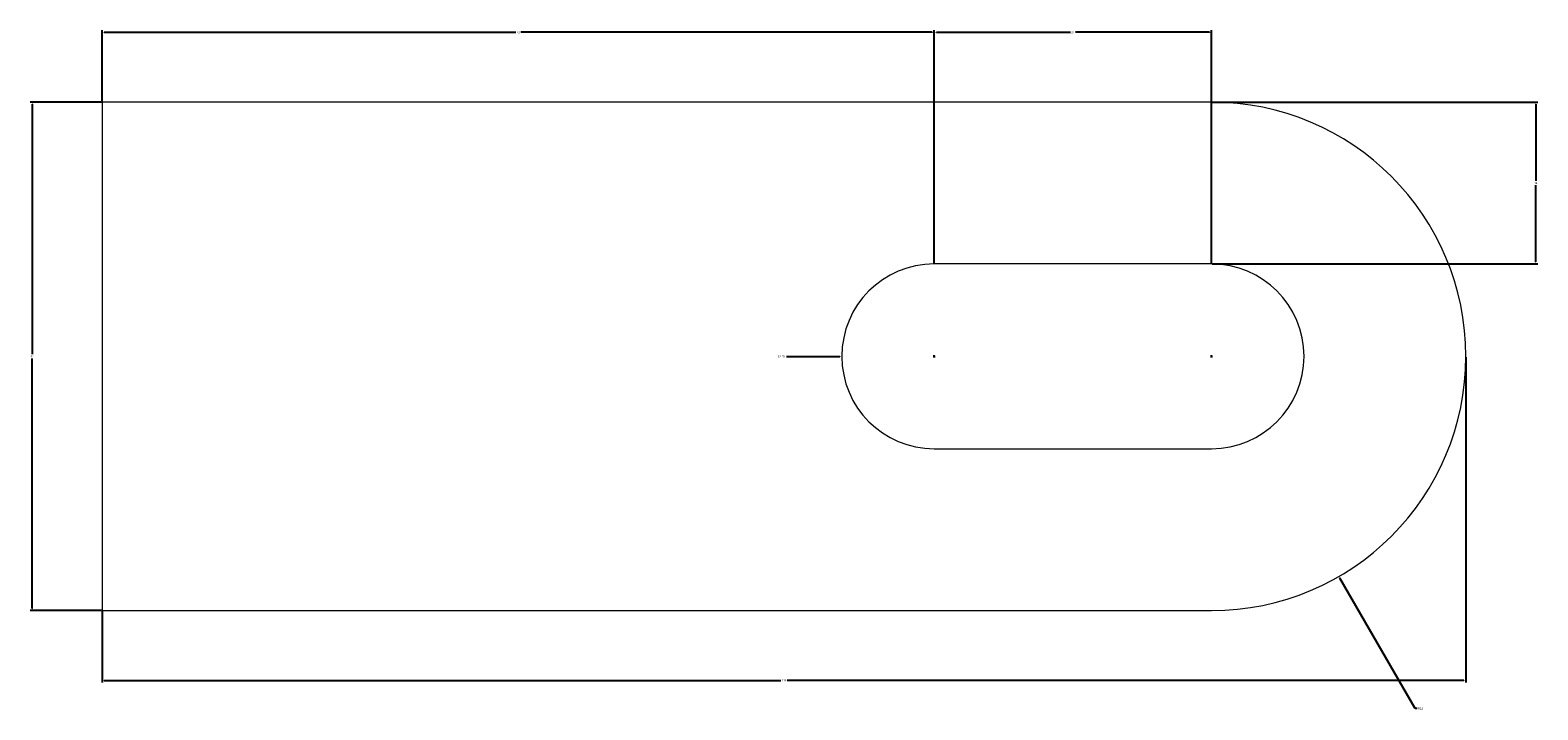
# Model space of a CAD drawing. Units: millimetres. Extents: x 3613 to 3838, y -3 to 1390.
# Tile 2 of 2: x 3613 to 3744, y 1331 to 1390. Entities that reach past the tile are written whole.
import ezdxf

# ---------------------------------------------------------------- set-up
doc = ezdxf.new("R2010")
doc.units = ezdxf.units.MM
doc.layers.add('M-CONS', color=7, linetype='Continuous', lineweight=18)
doc.layers.add('M-DIMS', color=2, linetype='Continuous', lineweight=18)
doc.styles.get("Standard").update_dxf_attribs({"font": 'arial.ttf'})
doc.dimstyles.get("Standard").update_dxf_attribs({"dimtxt": 0.18, "dimasz": 0.18, "dimexe": 0.18, "dimexo": 0.0625, "dimgap": 0.09, "dimtad": 0, "dimtih": 1, "dimtoh": 1, "dimdec": 4, "dimzin": 0, "dimdsep": 46, "dimtxsty": 'Standard', "dimcen": 0.09, "dimadec": 0, "dimazin": 0, "dimtfac": 1, "dimtdec": 4, "dimtofl": 0, "dimtmove": 0, "dimatfit": 3, "dimfxl": 1, "dimtolj": 1, "dimtzin": 0, "dimarcsym": 0})

# ---------------------------------------------------------------- blocks, each defined once
blk = doc.blocks.new('*D1')
at = {"layer": 'Defpoints', "color": 0, "transparency": 16777216}
for p in [(3737.71, 1361.28), (3619.71, 1339.28), (3737.71, 1333.23)]:
    blk.add_point(p, dxfattribs=at)
at = {"layer": 'M-DIMS', "color": 0, "lineweight": -2, "transparency": 16777216}
for p, q in [((3737.71, 1361.22), (3737.71, 1333.05)), ((3619.71, 1339.22), (3619.71, 1333.05)), ((3619.89, 1333.23), (3678.43, 1333.23)), ((3737.53, 1333.23), (3678.99, 1333.23))]:
    blk.add_line(p, q, dxfattribs=at)
at = {"layer": 'M-DIMS', "color": 0, "transparency": 16777216}
for points in [[(3619.89, 1333.26), (3619.89, 1333.2), (3619.71, 1333.23)], [(3737.53, 1333.26), (3737.53, 1333.2), (3737.71, 1333.23)]]:
    blk.add_solid(points, dxfattribs=at)
at = {"layer": 'M-DIMS', "color": 0, "transparency": 16777216, "insert": (3678.71, 1333.23), "char_height": 0.18, "attachment_point": 5}
blk.add_mtext('\\A1;118', dxfattribs=at)
blk = doc.blocks.new('*D2')
at = {"layer": 'Defpoints', "color": 0, "transparency": 16777216}
for p in [(3613.65792, 1383.283895), (3619.70792, 1383.283895), (3619.70792, 1339.283895)]:
    blk.add_point(p, dxfattribs=at)
at = {"layer": 'M-DIMS', "color": 0, "lineweight": -2, "transparency": 16777216}
for p, q in [((3619.64542, 1383.283895), (3613.47792, 1383.283895)), ((3613.65792, 1383.103895), (3613.65792, 1361.463895)), ((3613.65792, 1339.463895), (3613.65792, 1361.103895)), ((3619.64542, 1339.283895), (3613.47792, 1339.283895))]:
    blk.add_line(p, q, dxfattribs=at)
at = {"layer": 'M-DIMS', "color": 0, "transparency": 16777216}
for points in [[(3613.62792, 1383.103895), (3613.68792, 1383.103895), (3613.65792, 1383.283895)], [(3613.62792, 1339.463895), (3613.68792, 1339.463895), (3613.65792, 1339.283895)]]:
    blk.add_solid(points, dxfattribs=at)
at = {"layer": 'M-DIMS', "color": 0, "transparency": 16777216, "insert": (3613.65792, 1361.283895), "char_height": 0.18, "attachment_point": 5}
blk.add_mtext('\\A1;44', dxfattribs=at)
blk = doc.blocks.new('*D3')
at = {"layer": 'Defpoints', "color": 0, "transparency": 16777216}
for p in [(3715.71, 1389.33), (3691.71, 1369.28), (3715.71, 1369.28)]:
    blk.add_point(p, dxfattribs=at)
at = {"layer": 'M-DIMS', "color": 0, "lineweight": -2, "transparency": 16777216}
for p, q in [((3691.71, 1369.35), (3691.71, 1389.51)), ((3715.71, 1369.35), (3715.71, 1389.51)), ((3691.89, 1389.33), (3703.49, 1389.33)), ((3715.53, 1389.33), (3703.93, 1389.33))]:
    blk.add_line(p, q, dxfattribs=at)
at = {"layer": 'M-DIMS', "color": 0, "transparency": 16777216}
for points in [[(3691.89, 1389.36), (3691.89, 1389.3), (3691.71, 1389.33)], [(3715.53, 1389.36), (3715.53, 1389.3), (3715.71, 1389.33)]]:
    blk.add_solid(points, dxfattribs=at)
at = {"layer": 'M-DIMS', "color": 0, "transparency": 16777216, "insert": (3703.71, 1389.33), "char_height": 0.18, "attachment_point": 5}
blk.add_mtext('\\A1;24', dxfattribs=at)
blk = doc.blocks.new('*D4')
at = {"layer": 'Defpoints', "color": 0, "transparency": 16777216}
for p in [(3715.71, 1383.28), (3743.76, 1383.28), (3715.71, 1369.28)]:
    blk.add_point(p, dxfattribs=at)
at = {"layer": 'M-DIMS', "color": 0, "lineweight": -2, "transparency": 16777216}
for p, q in [((3715.77, 1383.28), (3743.94, 1383.28)), ((3743.76, 1383.1), (3743.76, 1376.46)), ((3743.76, 1369.46), (3743.76, 1376.1)), ((3715.77, 1369.28), (3743.94, 1369.28))]:
    blk.add_line(p, q, dxfattribs=at)
at = {"layer": 'M-DIMS', "color": 0, "transparency": 16777216}
for points in [[(3743.73, 1383.1), (3743.79, 1383.1), (3743.76, 1383.28)], [(3743.73, 1369.46), (3743.79, 1369.46), (3743.76, 1369.28)]]:
    blk.add_solid(points, dxfattribs=at)
at = {"layer": 'M-DIMS', "color": 0, "transparency": 16777216, "insert": (3743.76, 1376.28), "char_height": 0.18, "attachment_point": 5}
blk.add_mtext('\\A1;14', dxfattribs=at)
blk = doc.blocks.new('*D5')
at = {"layer": 'Defpoints', "color": 0, "transparency": 16777216}
for p in [(3691.71, 1389.33), (3619.71, 1383.28), (3691.71, 1369.28)]:
    blk.add_point(p, dxfattribs=at)
at = {"layer": 'M-DIMS', "color": 0, "lineweight": -2, "transparency": 16777216}
for p, q in [((3619.71, 1383.35), (3619.71, 1389.51)), ((3691.71, 1369.35), (3691.71, 1389.51)), ((3619.89, 1389.33), (3655.49, 1389.33)), ((3691.53, 1389.33), (3655.93, 1389.33))]:
    blk.add_line(p, q, dxfattribs=at)
at = {"layer": 'M-DIMS', "color": 0, "transparency": 16777216}
for points in [[(3619.89, 1389.36), (3619.89, 1389.3), (3619.71, 1389.33)], [(3691.53, 1389.36), (3691.53, 1389.3), (3691.71, 1389.33)]]:
    blk.add_solid(points, dxfattribs=at)
at = {"layer": 'M-DIMS', "color": 0, "transparency": 16777216, "insert": (3655.71, 1389.33), "char_height": 0.18, "attachment_point": 5}
blk.add_mtext('\\A1;72', dxfattribs=at)
blk = doc.blocks.new('*D7')
at = {"layer": 'Defpoints', "color": 0, "transparency": 16777216}
for p in [(3715.71, 1361.28), (3726.71, 1342.23)]:
    blk.add_point(p, dxfattribs=at)
at = {"layer": 'M-DIMS', "color": 0, "lineweight": -2, "transparency": 16777216}
for p, q in [((3715.62, 1361.28), (3715.8, 1361.28)), ((3715.71, 1361.19), (3715.71, 1361.37)), ((3733.31, 1330.8), (3726.8, 1342.08)), ((3733.49, 1330.8), (3733.31, 1330.8))]:
    blk.add_line(p, q, dxfattribs=at)
at = {"layer": 'M-DIMS', "color": 0, "transparency": 16777216}
blk.add_solid([(3726.82, 1342.09), (3726.77, 1342.06), (3726.71, 1342.23)], dxfattribs=at)
at = {"layer": 'M-DIMS', "color": 0, "transparency": 16777216, "insert": (3733.79, 1330.8), "char_height": 0.18, "attachment_point": 5}
blk.add_mtext('\\A1;R22', dxfattribs=at)
blk = doc.blocks.new('*D8')
at = {"layer": 'Defpoints', "color": 0, "transparency": 16777216}
for p in [(3683.71, 1361.28), (3691.71, 1361.28)]:
    blk.add_point(p, dxfattribs=at)
at = {"layer": 'M-DIMS', "color": 0, "lineweight": -2, "transparency": 16777216}
for p, q in [((3678.91, 1361.28), (3683.53, 1361.28)), ((3691.62, 1361.28), (3691.8, 1361.28)), ((3691.71, 1361.19), (3691.71, 1361.37))]:
    blk.add_line(p, q, dxfattribs=at)
at = {"layer": 'M-DIMS', "color": 0, "transparency": 16777216}
blk.add_solid([(3683.53, 1361.31), (3683.53, 1361.25), (3683.71, 1361.28)], dxfattribs=at)
at = {"layer": 'M-DIMS', "color": 0, "transparency": 16777216, "insert": (3678.48, 1361.28), "char_height": 0.18, "attachment_point": 5}
blk.add_mtext('\\A1;2X R8', dxfattribs=at)

msp = doc.modelspace()

# ---------------------------------------------------------------- linework, layer by layer
at = {"layer": 'M-CONS'}
for points in [[(3715.71, 1383.28), (3619.71, 1383.28), (3619.71, 1339.28), (3715.71, 1339.28, 1)], [(3715.71, 1369.28), (3691.71, 1369.28, 1), (3691.71, 1353.28), (3715.71, 1353.28, 1)]]:
    msp.add_lwpolyline(points, format="xyb", close=True, dxfattribs=at)

# ---------------------------------------------------------------- dimensions: what is measured, and where the dimension line sits
at = {"layer": 'M-DIMS'}
for base, p1, p2, picture, middle in [((3691.71, 1389.33), (3619.71, 1383.28), (3691.71, 1369.28), '*D5', (3655.71, 1389.33)), ((3715.71, 1389.33), (3691.71, 1369.28), (3715.71, 1369.28), '*D3', (3703.71, 1389.33)), ((3737.71, 1333.23), (3619.71, 1339.28), (3737.71, 1361.28), '*D1', (3678.71, 1333.23))]:
    dim = msp.add_linear_dim(base=base, p1=p1, p2=p2, dimstyle='Standard', override={"dimdec": 0, "dimlfac": 1, "dimrnd": 0, "dimzin": 0, "dimdsep": 46, "dimlunit": 2}, dxfattribs=at)
    dim.commit()
    dim.dimension.update_dxf_attribs({"geometry": picture, "text_midpoint": middle})
for base, p1, p2, picture, middle in [((3613.66, 1383.28), (3619.71, 1339.28), (3619.71, 1383.28), '*D2', (3613.66, 1361.28)), ((3743.76, 1383.28), (3715.71, 1369.28), (3715.71, 1383.28), '*D4', (3743.76, 1376.28))]:
    dim = msp.add_linear_dim(base=base, p1=p1, p2=p2, angle=90, dimstyle='Standard', override={"dimdec": 0, "dimlfac": 1, "dimrnd": 0, "dimzin": 0, "dimdsep": 46, "dimlunit": 2}, dxfattribs=at)
    dim.commit()
    dim.dimension.update_dxf_attribs({"geometry": picture, "text_midpoint": middle})
dim = msp.add_radius_dim(center=(3691.71, 1361.28), mpoint=(3683.71, 1361.28), text='2X <>', dimstyle='Standard', override={"dimdec": 0, "dimlfac": 1, "dimrnd": 0, "dimzin": 0, "dimdsep": 46, "dimlunit": 2}, dxfattribs=at)
dim.commit()
dim.dimension.update_dxf_attribs({"geometry": '*D8', "text_midpoint": (3678.91, 1361.28), "dimtype": 164})
dim = msp.add_radius_dim(center=(3715.71, 1361.28), mpoint=(3726.71, 1342.23), dimstyle='Standard', override={"dimdec": 0, "dimlfac": 1, "dimrnd": 0, "dimzin": 0, "dimdsep": 46, "dimlunit": 2}, dxfattribs=at)
dim.commit()
dim.dimension.update_dxf_attribs({"geometry": '*D7', "text_midpoint": (3733.79, 1330.8), "dimtype": 164})

doc.saveas('drawing.dxf')
